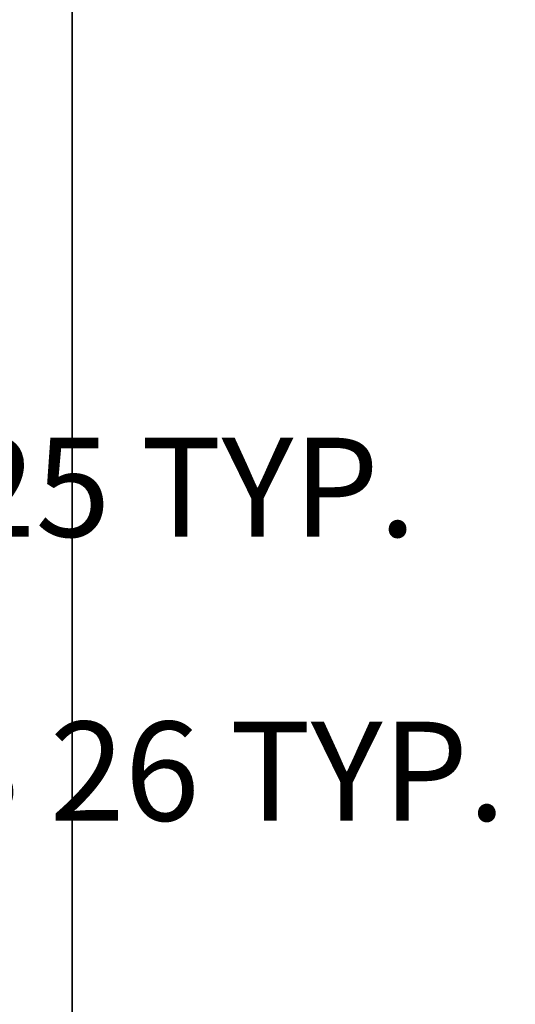
# Model space of a CAD drawing. Units: inches. Extents: x 1704 to 6393, y -157 to 1172.
# Tile 95 of 122: x 2720 to 2750, y 912 to 972. Entities that reach past the tile are written whole.
import ezdxf

# ---------------------------------------------------------------- set-up
doc = ezdxf.new("R2010")
doc.units = ezdxf.units.IN
doc.header["$MEASUREMENT"] = 0
doc.layers.add('A-ANNO-DIMS', color=7, linetype='Continuous', lineweight=13)
doc.layers.add('C-PROP', color=7, linetype='Continuous', lineweight=35)
doc.styles.get("Standard").update_dxf_attribs({"font": 'arial.ttf'})
doc.dimstyles.get("Standard").update_dxf_attribs({"dimtxt": 6, "dimasz": 2, "dimexe": 0.18, "dimexo": 0.0625, "dimgap": 0.09, "dimtad": 0, "dimtih": 1, "dimtoh": 1, "dimdec": 1, "dimzin": 0, "dimdsep": 46, "dimlunit": 3, "dimtxsty": 'Standard', "dimblk": 'ARCHTICK', "dimcen": 0.09, "dimadec": 0, "dimazin": 0, "dimtfac": 1, "dimtdec": 1, "dimtofl": 0, "dimtmove": 0, "dimatfit": 3, "dimfxl": 1, "dimtolj": 1, "dimtzin": 0, "dimarcsym": 0})

# ---------------------------------------------------------------- blocks, each defined once
blk = doc.blocks.new('_ArchTick')
at = {"color": 0, "linetype": 'ByBlock', "const_width": 0.15}
blk.add_lwpolyline([(-0.5, -0.5), (0.5, 0.5)], dxfattribs=at)
blk = doc.blocks.new('*D84')
at = {"layer": 'A-ANNO-DIMS', "color": 0, "lineweight": -2, "transparency": 16777216}
for p, q in [((2713.724, 939.698), (2717.812, 939.698)), ((2717.632, 939.698), (2717.632, 929.658)), ((2717.632, 913.234), (2717.632, 923.274)), ((2713.724, 913.234), (2717.812, 913.234))]:
    blk.add_line(p, q, dxfattribs=at)
at = {"layer": 'Defpoints', "color": 0, "lineweight": -3, "transparency": 16777216}
for p in [(2713.662, 939.698), (2713.662, 913.234), (2717.632, 913.234)]:
    blk.add_point(p, dxfattribs=at)
at = {"layer": 'A-ANNO-DIMS', "color": 0, "lineweight": -2, "transparency": 16777216, "xscale": 2, "yscale": 2, "zscale": 2}
for p, rotation in [((2717.632, 939.698), 90), ((2717.632, 913.234), 270)]:
    blk.add_blockref('_ArchTick', p, dxfattribs=dict(at, rotation=rotation))
at = {"layer": 'A-ANNO-DIMS', "color": 0, "transparency": 16777216, "insert": (2717.632, 926.466), "char_height": 6, "attachment_point": 5}
blk.add_mtext('\\A1;SHRUB B 26 TYP.', dxfattribs=at)
blk = doc.blocks.new('*D85')
at = {"layer": 'A-ANNO-DIMS', "color": 0, "lineweight": -2, "transparency": 16777216}
for p, q in [((2688.434, 939.761), (2688.434, 943.848)), ((2713.662, 939.761), (2713.662, 943.848)), ((2688.434, 943.668), (2713.662, 943.668)), ((2713.662, 943.668), (2715.662, 943.668))]:
    blk.add_line(p, q, dxfattribs=at)
at = {"layer": 'Defpoints', "color": 0, "lineweight": -3, "transparency": 16777216}
for p in [(2713.662, 943.668), (2688.434, 939.698), (2713.662, 939.698)]:
    blk.add_point(p, dxfattribs=at)
at = {"layer": 'A-ANNO-DIMS', "color": 0, "lineweight": -2, "transparency": 16777216, "xscale": 2, "yscale": 2, "zscale": 2, "rotation": 180}
blk.add_blockref('_ArchTick', (2688.434, 943.668), dxfattribs=at)
at = {"layer": 'A-ANNO-DIMS', "color": 0, "lineweight": -2, "transparency": 16777216, "xscale": 2, "yscale": 2, "zscale": 2}
blk.add_blockref('_ArchTick', (2713.662, 943.668), dxfattribs=at)
at = {"layer": 'A-ANNO-DIMS', "color": 0, "transparency": 16777216, "insert": (2730.406, 943.668), "char_height": 6, "attachment_point": 5}
blk.add_mtext('\\A1;25 TYP.', dxfattribs=at)
blk = doc.blocks.new('*D91')
at = {"layer": 'A-ANNO-DIMS', "color": 0, "lineweight": -2, "transparency": 16777216}
for p, q in [((2723.411, 1033.213), (2784.529, 1033.213)), ((2784.349, 1033.213), (2784.349, 517.868)), ((2784.349, -3.787), (2784.349, 511.557)), ((2723.411, -3.787), (2784.529, -3.787))]:
    blk.add_line(p, q, dxfattribs=at)
at = {"layer": 'Defpoints', "color": 0, "lineweight": -3, "transparency": 16777216}
for p in [(2723.349, 1033.213), (2784.349, 1033.213), (2723.349, -3.787)]:
    blk.add_point(p, dxfattribs=at)
at = {"layer": 'A-ANNO-DIMS', "color": 0, "lineweight": -2, "transparency": 16777216, "xscale": 2, "yscale": 2, "zscale": 2}
for p, rotation in [((2784.349, 1033.213), 90), ((2784.349, -3.787), 270)]:
    blk.add_blockref('_ArchTick', p, dxfattribs=dict(at, rotation=rotation))
at = {"layer": 'A-ANNO-DIMS', "color": 0, "transparency": 16777216, "insert": (2784.349, 514.713), "char_height": 6, "attachment_point": 5}
blk.add_mtext('\\A1;1037', dxfattribs=at)
blk = doc.blocks.new('*D95')
at = {"layer": 'A-ANNO-DIMS', "color": 0, "lineweight": -2, "transparency": 16777216}
for p, q in [((2605.349, 895.275), (2605.349, 1105.287)), ((2605.349, 1105.107), (2657.907, 1105.107)), ((2723.349, 1105.107), (2670.791, 1105.107)), ((2723.349, 895.275), (2723.349, 1105.287))]:
    blk.add_line(p, q, dxfattribs=at)
at = {"layer": 'Defpoints', "color": 0, "lineweight": -3, "transparency": 16777216}
for p in [(2723.349, 1105.107), (2605.349, 895.213), (2723.349, 895.213)]:
    blk.add_point(p, dxfattribs=at)
at = {"layer": 'A-ANNO-DIMS', "color": 0, "lineweight": -2, "transparency": 16777216, "xscale": 2, "yscale": 2, "zscale": 2, "rotation": 180}
blk.add_blockref('_ArchTick', (2605.349, 1105.107), dxfattribs=at)
at = {"layer": 'A-ANNO-DIMS', "color": 0, "lineweight": -2, "transparency": 16777216, "xscale": 2, "yscale": 2, "zscale": 2}
blk.add_blockref('_ArchTick', (2723.349, 1105.107), dxfattribs=at)
at = {"layer": 'A-ANNO-DIMS', "color": 0, "transparency": 16777216, "insert": (2664.349, 1105.107), "char_height": 6, "attachment_point": 5}
blk.add_mtext('\\A1;118', dxfattribs=at)

msp = doc.modelspace()

# ---------------------------------------------------------------- linework, layer by layer
at = {"layer": 'C-PROP'}
msp.add_line((2723.349, -3.787), (2723.349, 1033.213), dxfattribs=at)

# ---------------------------------------------------------------- dimensions: what is measured, and where the dimension line sits
at = {"layer": 'A-ANNO-DIMS'}
dim = msp.add_linear_dim(base=(2723.349, 1105.107), p1=(2605.349, 895.213), p2=(2723.349, 895.213), dimstyle='Standard', override={"dimdec": 0, "dimlfac": 1, "dimrnd": 0, "dimzin": 0, "dimdsep": 46, "dimlunit": 2}, dxfattribs=at)
dim.commit()
dim.dimension.update_dxf_attribs({"geometry": '*D95', "text_midpoint": (2664.349, 1105.107)})
dim = msp.add_linear_dim(base=(2784.349, 1033.213), p1=(2723.349, -3.787), p2=(2723.349, 1033.213), angle=90, dimstyle='Standard', override={"dimdec": 0, "dimlfac": 1, "dimrnd": 0, "dimzin": 0, "dimdsep": 46, "dimlunit": 2}, dxfattribs=at)
dim.commit()
dim.dimension.update_dxf_attribs({"geometry": '*D91', "text_midpoint": (2784.349, 514.713)})
dim = msp.add_linear_dim(base=(2713.662, 943.668), p1=(2688.434, 939.698), p2=(2713.662, 939.698), text='<> TYP.', dimstyle='Standard', override={"dimdec": 0, "dimlfac": 1, "dimrnd": 0, "dimzin": 0, "dimdsep": 46, "dimlunit": 2}, dxfattribs=at)
dim.commit()
dim.dimension.update_dxf_attribs({"geometry": '*D85', "text_midpoint": (2730.406, 943.668)})
dim = msp.add_linear_dim(base=(2717.632, 913.234), p1=(2713.662, 939.698), p2=(2713.662, 913.234), angle=270, text='SHRUB B <> TYP.', dimstyle='Standard', override={"dimdec": 0, "dimlfac": 1, "dimrnd": 0, "dimzin": 0, "dimdsep": 46, "dimlunit": 2}, dxfattribs=at)
dim.commit()
dim.dimension.update_dxf_attribs({"geometry": '*D84', "text_midpoint": (2717.632, 926.466)})

doc.saveas('drawing.dxf')
